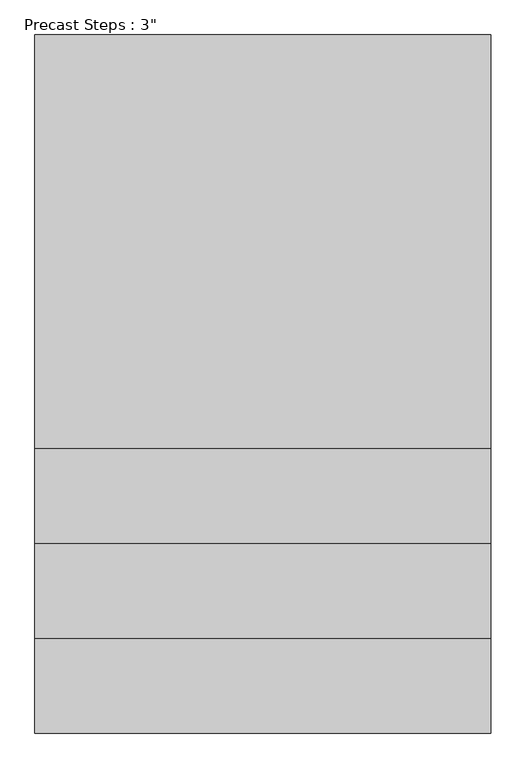
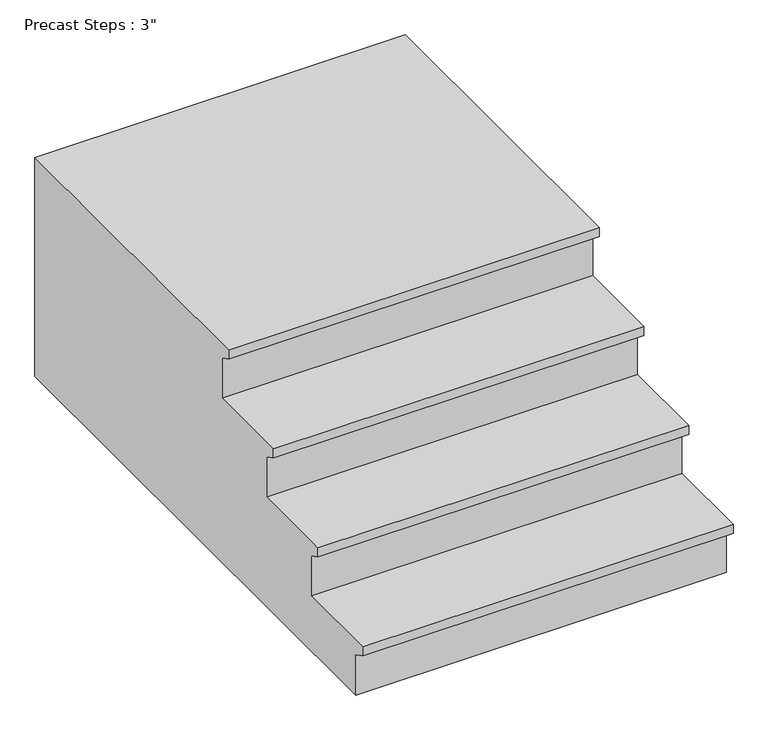
"""IFC4 building model written with IfcOpenShell, lengths in millimetres: geographic element geometry."""

from ifc_helpers import new_model, si_unit, frame, origin, place, context, project, spatial, polyline, outline, extrude, source, transform, mapped, element, save


def geographic_element_a8b2e6db(model_context):
    return source(origin(), model_context, "Body", "SweptSolid", [
        extrude(outline(polyline([(0.0, 762.0), (0.0, 0.0), (-1828.8, 0.0), (-1828.8, 139.7), (-1866.9, 159.2389913), (-1866.9, 190.5), (-1574.8, 190.5), (-1574.8, 330.2), (-1612.9, 349.7389913), (-1612.9, 381.0), (-1320.8, 381.0), (-1320.8, 520.7), (-1358.9, 540.2389913), (-1358.9, 571.5), (-1066.8, 571.5), (-1066.8, 711.2), (-1104.9, 730.7389913), (-1104.9, 762.0), (0.0, 762.0)])), frame((-638.9441956, 0.0, 0.0), z_axis=(1.0, 0.0, 0.0), x_axis=(0.0, 1.0, 0.0)), (0.0, 0.0, 1.0), 1219.2),
    ])


if __name__ == "__main__":
    model = new_model("IFC4")
    model_context = context("Model", 3, world=origin())
    ifc_project = project(units=[si_unit("LENGTHUNIT", "METRE", prefix="MILLI")], contexts=[model_context])
    site = spatial("IfcSite", under=ifc_project)
    building = spatial("IfcBuilding", under=site)
    placement = place(None, origin())
    geographic_element_shape = geographic_element_a8b2e6db(model_context)
    element("IfcGeographicElement", 1, ObjectType="Precast Steps : 3\"", at=placement, inside=building, context=model_context, shape_type="MappedRepresentation", body=[
        mapped(geographic_element_shape, transform((0.0, 0.0, 0.0), x_axis=(1.0, 0.0, 0.0), y_axis=(0.0, 1.0, 0.0), z_axis=(0.0, 0.0, 1.0))),
    ])
    save(model, "model.ifc")

# Revit data of these elements
# Type "Precast Steps : 3\""
#   Assembly Code = "G"
#   Landing = 3' - 6"
#   Step Offset = 0' - 10"
#   Width = 4' - 0"
#   Material = Concrete - Precast Concrete
# Element 1 (IfcGeographicElement, "Precast Steps : 3\"")
#   Materials on its faces: "Concrete - Precast Concrete"
# Materials
#   "Concrete - Precast Concrete": colour RGB 198 187 187, transparency 0
